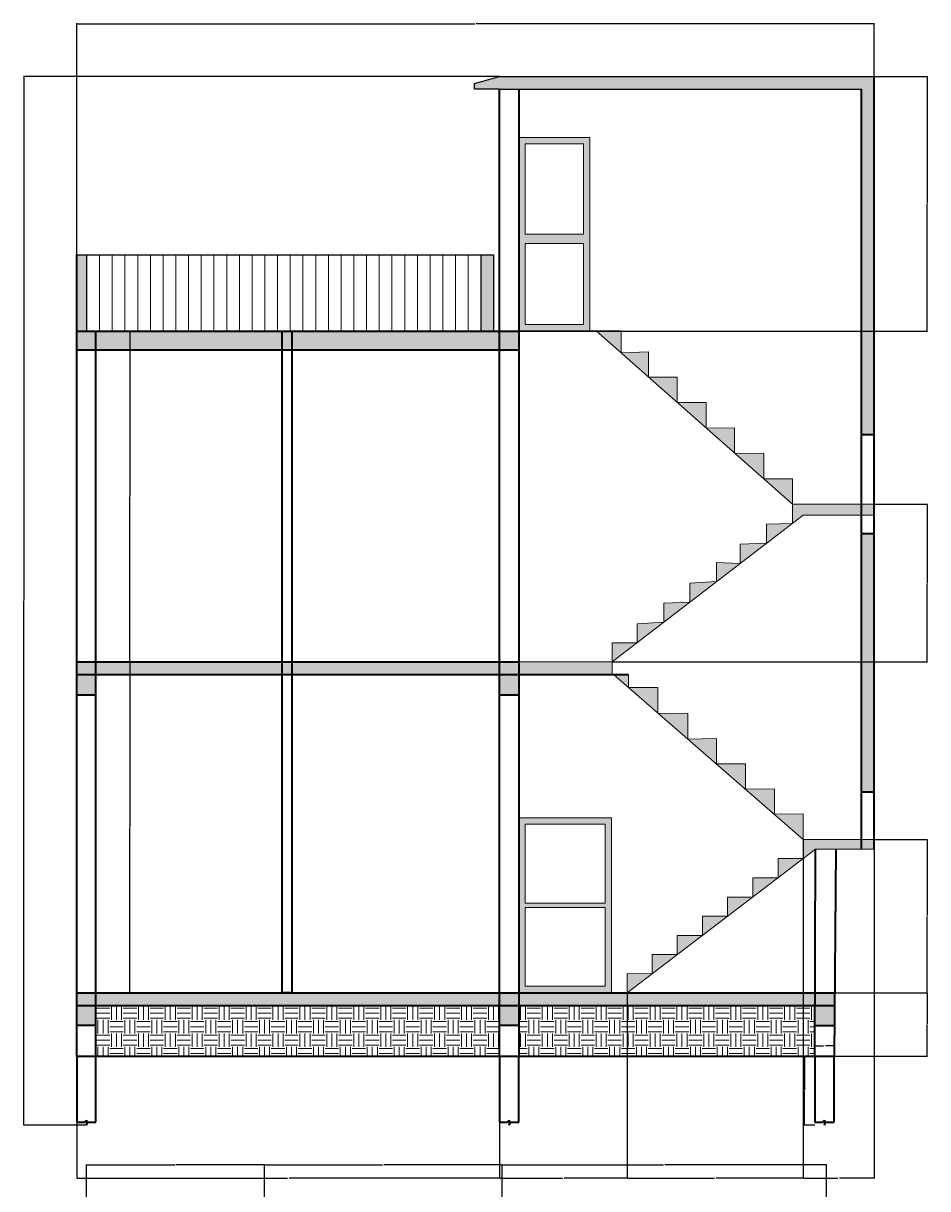
# Model space of a CAD drawing. Units: inches. Extents: x 3504 to 4623, y 2365 to 3357.
# Tile 5 of 5: x 4131 to 4558, y 2803 to 3352. Entities that reach past the tile are written whole.
import ezdxf

# ---------------------------------------------------------------- set-up
doc = ezdxf.new("R2010")
doc.units = ezdxf.units.IN
for name, color, linetype, lineweight in [('A-ANNO-DIMS', 2, 'Continuous', 18), ('A-DOOR', 3, 'Continuous', 18), ('A-FLOR-HRAL', 7, 'Continuous', 25), ('A-FLOR-HRAL-PATT', 252, 'Continuous', 13), ('A-FLOR-STRS', 7, 'Continuous', 18), ('A-ROOF', 7, 'Continuous', 25), ('A-SECT', 7, 'Continuous', 35), ('S-FNDN', 7, 'Continuous', 35)]:
    doc.layers.add(name, color=color, linetype=linetype, lineweight=lineweight)
doc.layers.add('A-SECT-PATT', color=9, linetype='Continuous', lineweight=13, true_color=0xc7c8ca)
doc.layers.add('S-FNDN-PATT', color=9, linetype='Continuous', lineweight=13, true_color=0xc7c8ca)
doc.styles.get("Standard").update_dxf_attribs({"font": 'arial.ttf'})
doc.dimstyles.get("Standard").update_dxf_attribs({"dimtxt": 0.18, "dimasz": 0.18, "dimexe": 0.18, "dimexo": 0.0625, "dimgap": 0.09, "dimtad": 0, "dimtih": 1, "dimtoh": 1, "dimdec": 4, "dimzin": 0, "dimdsep": 46, "dimtxsty": 'Standard', "dimcen": 0.09, "dimadec": 0, "dimazin": 0, "dimtfac": 1, "dimtdec": 4, "dimtofl": 0, "dimtmove": 0, "dimatfit": 3, "dimfxl": 1, "dimtolj": 1, "dimtzin": 0, "dimarcsym": 0})

# ---------------------------------------------------------------- blocks, each defined once
blk = doc.blocks.new('PIER-9-BROKEN-SECTION')
for p, q in [((0, 32.48), (0, 1.39)), ((9, 1.39), (9, 32.48)), ((0, 1.39), (3.55, 1.39)), ((3.55, 1.39), (4.5, 2.34)), ((4.5, 2.34), (4.5, 0)), ((4.5, 0), (5.04, 1.39)), ((5.04, 1.39), (9, 1.39))]:
    blk.add_line(p, q)
blk = doc.blocks.new('*D23')
at = {"layer": 'A-ANNO-DIMS', "color": 0, "lineweight": -2, "transparency": 16777216}
for p, q in [((4504.48, 2864.98), (4499.49, 2864.98)), ((4499.67, 2864.8), (4499.67, 2848.93)), ((4499.67, 2832.69), (4499.67, 2848.56)), ((4504.48, 2832.51), (4499.49, 2832.51))]:
    blk.add_line(p, q, dxfattribs=at)
at = {"layer": 'A-ANNO-DIMS', "color": 0, "transparency": 16777216}
for points in [[(4499.64, 2864.8), (4499.7, 2864.8), (4499.67, 2864.98)], [(4499.64, 2832.69), (4499.7, 2832.69), (4499.67, 2832.51)]]:
    blk.add_solid(points, dxfattribs=at)
at = {"layer": 'Defpoints', "color": 0, "transparency": 16777216}
for p in [(4499.67, 2864.98), (4504.54, 2864.98), (4504.54, 2832.51)]:
    blk.add_point(p, dxfattribs=at)
at = {"layer": 'A-ANNO-DIMS', "color": 0, "transparency": 16777216, "insert": (4499.67, 2848.74), "char_height": 0.18, "attachment_point": 5}
blk.add_mtext('\\A1;PIER 32 TYP.', dxfattribs=at)
blk = doc.blocks.new('*D24')
at = {"layer": 'A-ANNO-DIMS', "color": 0, "lineweight": -2, "transparency": 16777216}
for p, q in [((4504.54, 2865.05), (4504.54, 2870.04)), ((4504.72, 2869.86), (4508.58, 2869.86)), ((4513.36, 2869.86), (4509.5, 2869.86)), ((4513.54, 2865.05), (4513.54, 2870.04))]:
    blk.add_line(p, q, dxfattribs=at)
at = {"layer": 'A-ANNO-DIMS', "color": 0, "transparency": 16777216}
for points in [[(4504.72, 2869.89), (4504.72, 2869.83), (4504.54, 2869.86)], [(4513.36, 2869.89), (4513.36, 2869.83), (4513.54, 2869.86)]]:
    blk.add_solid(points, dxfattribs=at)
at = {"layer": 'Defpoints', "color": 0, "transparency": 16777216}
for p in [(4513.54, 2869.86), (4504.54, 2864.98), (4513.54, 2864.98)]:
    blk.add_point(p, dxfattribs=at)
at = {"layer": 'A-ANNO-DIMS', "color": 0, "transparency": 16777216, "insert": (4509.04, 2869.86), "char_height": 0.18, "attachment_point": 5}
blk.add_mtext('\\A1;9 TYP.', dxfattribs=at)
blk = doc.blocks.new('*D37')
at = {"layer": 'A-ANNO-DIMS', "color": 0, "lineweight": -2, "transparency": 16777216}
for p, q in [((4160.95, 2788.12), (4160.95, 2813.99)), ((4161.13, 2813.81), (4202.73, 2813.81)), ((4244.77, 2813.81), (4203.17, 2813.81)), ((4244.95, 2788.12), (4244.95, 2813.99))]:
    blk.add_line(p, q, dxfattribs=at)
at = {"layer": 'A-ANNO-DIMS', "color": 0, "transparency": 16777216}
for points in [[(4161.13, 2813.84), (4161.13, 2813.78), (4160.95, 2813.81)], [(4244.77, 2813.84), (4244.77, 2813.78), (4244.95, 2813.81)]]:
    blk.add_solid(points, dxfattribs=at)
at = {"layer": 'Defpoints', "color": 0, "transparency": 16777216}
for p in [(4244.95, 2813.81), (4160.95, 2788.06), (4244.95, 2788.06)]:
    blk.add_point(p, dxfattribs=at)
at = {"layer": 'A-ANNO-DIMS', "color": 0, "transparency": 16777216, "insert": (4202.95, 2813.81), "char_height": 0.18, "attachment_point": 5}
blk.add_mtext('\\A1;84', dxfattribs=at)
blk = doc.blocks.new('*D38')
at = {"layer": 'A-ANNO-DIMS', "color": 0, "lineweight": -2, "transparency": 16777216}
for p, q in [((4244.95, 2788.12), (4244.95, 2813.99)), ((4245.13, 2813.81), (4300.67, 2813.81)), ((4356.77, 2813.81), (4301.23, 2813.81)), ((4356.95, 2788.12), (4356.95, 2813.99))]:
    blk.add_line(p, q, dxfattribs=at)
at = {"layer": 'A-ANNO-DIMS', "color": 0, "transparency": 16777216}
for points in [[(4245.13, 2813.84), (4245.13, 2813.78), (4244.95, 2813.81)], [(4356.77, 2813.84), (4356.77, 2813.78), (4356.95, 2813.81)]]:
    blk.add_solid(points, dxfattribs=at)
at = {"layer": 'Defpoints', "color": 0, "transparency": 16777216}
for p in [(4356.95, 2813.81), (4244.95, 2788.06), (4356.95, 2788.06)]:
    blk.add_point(p, dxfattribs=at)
at = {"layer": 'A-ANNO-DIMS', "color": 0, "transparency": 16777216, "insert": (4300.95, 2813.81), "char_height": 0.18, "attachment_point": 5}
blk.add_mtext('\\A1;112', dxfattribs=at)
blk = doc.blocks.new('*D39')
at = {"layer": 'A-ANNO-DIMS', "color": 0, "lineweight": -2, "transparency": 16777216}
for p, q in [((4356.95, 2788.12), (4356.95, 2813.99)), ((4357.13, 2813.81), (4433.17, 2813.81)), ((4509.77, 2813.81), (4433.73, 2813.81)), ((4509.95, 2788.12), (4509.95, 2813.99))]:
    blk.add_line(p, q, dxfattribs=at)
at = {"layer": 'A-ANNO-DIMS', "color": 0, "transparency": 16777216}
for points in [[(4357.13, 2813.84), (4357.13, 2813.78), (4356.95, 2813.81)], [(4509.77, 2813.84), (4509.77, 2813.78), (4509.95, 2813.81)]]:
    blk.add_solid(points, dxfattribs=at)
at = {"layer": 'Defpoints', "color": 0, "transparency": 16777216}
for p in [(4509.95, 2813.81), (4356.95, 2788.06), (4509.95, 2788.06)]:
    blk.add_point(p, dxfattribs=at)
at = {"layer": 'A-ANNO-DIMS', "color": 0, "transparency": 16777216, "insert": (4433.45, 2813.81), "char_height": 0.18, "attachment_point": 5}
blk.add_mtext('\\A1;153', dxfattribs=at)
blk = doc.blocks.new('*D64')
at = {"layer": 'A-ANNO-DIMS', "color": 0, "lineweight": -2, "transparency": 16777216}
for p, q in [((4156.45, 3243.05), (4156.45, 3352.11)), ((4156.63, 3351.93), (4344.16, 3351.93)), ((4532.27, 3351.93), (4344.74, 3351.93)), ((4532.45, 3327.05), (4532.45, 3352.11))]:
    blk.add_line(p, q, dxfattribs=at)
at = {"layer": 'A-ANNO-DIMS', "color": 0, "transparency": 16777216}
for points in [[(4156.63, 3351.96), (4156.63, 3351.9), (4156.45, 3351.93)], [(4532.27, 3351.96), (4532.27, 3351.9), (4532.45, 3351.93)]]:
    blk.add_solid(points, dxfattribs=at)
at = {"layer": 'Defpoints', "color": 0, "transparency": 16777216}
for p in [(4532.45, 3351.93), (4532.45, 3326.98), (4156.45, 3242.98)]:
    blk.add_point(p, dxfattribs=at)
at = {"layer": 'A-ANNO-DIMS', "color": 0, "transparency": 16777216, "insert": (4344.45, 3351.93), "char_height": 0.18, "attachment_point": 5}
blk.add_mtext('\\A1;376', dxfattribs=at)
blk = doc.blocks.new('*D65')
at = {"layer": 'A-ANNO-DIMS', "color": 0, "lineweight": -2, "transparency": 16777216}
for p, q in [((4355.78, 3326.98), (4131.32, 3326.98)), ((4131.5, 3326.8), (4131.5, 3079.93)), ((4131.5, 2832.69), (4131.5, 3079.56)), ((4160.89, 2832.51), (4131.32, 2832.51))]:
    blk.add_line(p, q, dxfattribs=at)
at = {"layer": 'A-ANNO-DIMS', "color": 0, "transparency": 16777216}
for points in [[(4131.47, 3326.8), (4131.53, 3326.8), (4131.5, 3326.98)], [(4131.47, 2832.69), (4131.53, 2832.69), (4131.5, 2832.51)]]:
    blk.add_solid(points, dxfattribs=at)
at = {"layer": 'Defpoints', "color": 0, "transparency": 16777216}
for p in [(4131.5, 3326.98), (4355.84, 3326.98), (4160.95, 2832.51)]:
    blk.add_point(p, dxfattribs=at)
at = {"layer": 'A-ANNO-DIMS', "color": 0, "transparency": 16777216, "insert": (4131.5, 3079.74), "char_height": 0.18, "attachment_point": 5}
blk.add_mtext('\\A1;494.5', dxfattribs=at)
blk = doc.blocks.new('*D66')
at = {"layer": 'A-ANNO-DIMS', "color": 0, "lineweight": -2, "transparency": 16777216}
for p, q in [((4513.88, 2894.98), (4557.58, 2894.98)), ((4557.4, 2894.8), (4557.4, 2880.17)), ((4557.4, 2865.16), (4557.4, 2879.8)), ((4513.6, 2864.98), (4557.58, 2864.98))]:
    blk.add_line(p, q, dxfattribs=at)
at = {"layer": 'A-ANNO-DIMS', "color": 0, "transparency": 16777216}
for points in [[(4557.37, 2894.8), (4557.43, 2894.8), (4557.4, 2894.98)], [(4557.37, 2865.16), (4557.43, 2865.16), (4557.4, 2864.98)]]:
    blk.add_solid(points, dxfattribs=at)
at = {"layer": 'Defpoints', "color": 0, "transparency": 16777216}
for p in [(4513.82, 2894.98), (4557.4, 2894.98), (4513.54, 2864.98)]:
    blk.add_point(p, dxfattribs=at)
at = {"layer": 'A-ANNO-DIMS', "color": 0, "transparency": 16777216, "insert": (4557.4, 2879.98), "char_height": 0.18, "attachment_point": 5}
blk.add_mtext('\\A1;30', dxfattribs=at)
blk = doc.blocks.new('*D67')
at = {"layer": 'A-ANNO-DIMS', "color": 0, "lineweight": -2, "transparency": 16777216}
for p, q in [((4532.51, 2967.25), (4557.58, 2967.25)), ((4557.4, 2967.07), (4557.4, 2931.3)), ((4557.4, 2895.16), (4557.4, 2930.94)), ((4513.88, 2894.98), (4557.58, 2894.98))]:
    blk.add_line(p, q, dxfattribs=at)
at = {"layer": 'A-ANNO-DIMS', "color": 0, "transparency": 16777216}
for points in [[(4557.37, 2967.07), (4557.43, 2967.07), (4557.4, 2967.25)], [(4557.37, 2895.16), (4557.43, 2895.16), (4557.4, 2894.98)]]:
    blk.add_solid(points, dxfattribs=at)
at = {"layer": 'Defpoints', "color": 0, "transparency": 16777216}
for p in [(4532.45, 2967.25), (4557.4, 2967.25), (4513.82, 2894.98)]:
    blk.add_point(p, dxfattribs=at)
at = {"layer": 'A-ANNO-DIMS', "color": 0, "transparency": 16777216, "insert": (4557.4, 2931.12), "char_height": 0.18, "attachment_point": 5}
blk.add_mtext('\\A1;72.27', dxfattribs=at)
blk = doc.blocks.new('*D68')
at = {"layer": 'A-ANNO-DIMS', "color": 0, "lineweight": -2, "transparency": 16777216}
for p, q in [((4156.51, 3050.98), (4181.58, 3050.98)), ((4181.4, 3050.8), (4181.4, 2973.17)), ((4181.4, 2895.16), (4181.4, 2972.8)), ((4156.51, 2894.98), (4181.58, 2894.98))]:
    blk.add_line(p, q, dxfattribs=at)
at = {"layer": 'A-ANNO-DIMS', "color": 0, "transparency": 16777216}
for points in [[(4181.37, 3050.8), (4181.43, 3050.8), (4181.4, 3050.98)], [(4181.37, 2895.16), (4181.43, 2895.16), (4181.4, 2894.98)]]:
    blk.add_solid(points, dxfattribs=at)
at = {"layer": 'Defpoints', "color": 0, "transparency": 16777216}
for p in [(4156.45, 3050.98), (4156.45, 2894.98), (4181.4, 2894.98)]:
    blk.add_point(p, dxfattribs=at)
at = {"layer": 'A-ANNO-DIMS', "color": 0, "transparency": 16777216, "insert": (4181.4, 2972.98), "char_height": 0.18, "attachment_point": 5}
blk.add_mtext('\\A1;156', dxfattribs=at)
blk = doc.blocks.new('*D69')
at = {"layer": 'A-ANNO-DIMS', "color": 0, "lineweight": -2, "transparency": 16777216}
for p, q in [((4156.51, 3206.98), (4181.58, 3206.98)), ((4181.4, 3206.8), (4181.4, 3129.17)), ((4181.4, 3051.16), (4181.4, 3128.8)), ((4156.51, 3050.98), (4181.58, 3050.98))]:
    blk.add_line(p, q, dxfattribs=at)
at = {"layer": 'A-ANNO-DIMS', "color": 0, "transparency": 16777216}
for points in [[(4181.37, 3206.8), (4181.43, 3206.8), (4181.4, 3206.98)], [(4181.37, 3051.16), (4181.43, 3051.16), (4181.4, 3050.98)]]:
    blk.add_solid(points, dxfattribs=at)
at = {"layer": 'Defpoints', "color": 0, "transparency": 16777216}
for p in [(4156.45, 3206.98), (4156.45, 3050.98), (4181.4, 3050.98)]:
    blk.add_point(p, dxfattribs=at)
at = {"layer": 'A-ANNO-DIMS', "color": 0, "transparency": 16777216, "insert": (4181.4, 3128.98), "char_height": 0.18, "attachment_point": 5}
blk.add_mtext('\\A1;156', dxfattribs=at)
blk = doc.blocks.new('*D70')
at = {"layer": 'A-ANNO-DIMS', "color": 0, "lineweight": -2, "transparency": 16777216}
for p, q in [((4532.51, 3125.28), (4557.58, 3125.28)), ((4557.4, 3125.1), (4557.4, 3088.31)), ((4557.4, 3051.16), (4557.4, 3087.95)), ((4408.96, 3050.98), (4557.58, 3050.98))]:
    blk.add_line(p, q, dxfattribs=at)
at = {"layer": 'A-ANNO-DIMS', "color": 0, "transparency": 16777216}
for points in [[(4557.37, 3125.1), (4557.43, 3125.1), (4557.4, 3125.28)], [(4557.37, 3051.16), (4557.43, 3051.16), (4557.4, 3050.98)]]:
    blk.add_solid(points, dxfattribs=at)
at = {"layer": 'Defpoints', "color": 0, "transparency": 16777216}
for p in [(4532.45, 3125.28), (4557.4, 3125.28), (4408.9, 3050.98)]:
    blk.add_point(p, dxfattribs=at)
at = {"layer": 'A-ANNO-DIMS', "color": 0, "transparency": 16777216, "insert": (4557.4, 3088.13), "char_height": 0.18, "attachment_point": 5}
blk.add_mtext('\\A1;74.3', dxfattribs=at)
blk = doc.blocks.new('*D71')
at = {"layer": 'A-ANNO-DIMS', "color": 0, "lineweight": -2, "transparency": 16777216}
for p, q in [((4532.51, 3326.98), (4557.58, 3326.98)), ((4557.4, 3326.8), (4557.4, 3267.17)), ((4557.4, 3207.16), (4557.4, 3266.8)), ((4364.91, 3206.98), (4557.58, 3206.98))]:
    blk.add_line(p, q, dxfattribs=at)
at = {"layer": 'A-ANNO-DIMS', "color": 0, "transparency": 16777216}
for points in [[(4557.37, 3326.8), (4557.43, 3326.8), (4557.4, 3326.98)], [(4557.37, 3207.16), (4557.43, 3207.16), (4557.4, 3206.98)]]:
    blk.add_solid(points, dxfattribs=at)
at = {"layer": 'Defpoints', "color": 0, "transparency": 16777216}
for p in [(4532.45, 3326.98), (4557.4, 3326.98), (4364.84, 3206.98)]:
    blk.add_point(p, dxfattribs=at)
at = {"layer": 'A-ANNO-DIMS', "color": 0, "transparency": 16777216, "insert": (4557.4, 3266.98), "char_height": 0.18, "attachment_point": 5}
blk.add_mtext('\\A1;120', dxfattribs=at)
blk = doc.blocks.new('*D72')
at = {"layer": 'A-ANNO-DIMS', "color": 0, "lineweight": -2, "transparency": 16777216}
for p, q in [((4156.45, 2833.83), (4156.45, 2807.38)), ((4355.84, 2833.83), (4355.84, 2807.38)), ((4156.63, 2807.56), (4255.76, 2807.56)), ((4355.66, 2807.56), (4256.53, 2807.56))]:
    blk.add_line(p, q, dxfattribs=at)
at = {"layer": 'A-ANNO-DIMS', "color": 0, "transparency": 16777216}
for points in [[(4156.63, 2807.59), (4156.63, 2807.53), (4156.45, 2807.56)], [(4355.66, 2807.59), (4355.66, 2807.53), (4355.84, 2807.56)]]:
    blk.add_solid(points, dxfattribs=at)
at = {"layer": 'Defpoints', "color": 0, "transparency": 16777216}
for p in [(4156.45, 2833.9), (4355.84, 2833.9), (4355.84, 2807.56)]:
    blk.add_point(p, dxfattribs=at)
at = {"layer": 'A-ANNO-DIMS', "color": 0, "transparency": 16777216, "insert": (4256.15, 2807.56), "char_height": 0.18, "attachment_point": 5}
blk.add_mtext('\\A1;199.4', dxfattribs=at)
blk = doc.blocks.new('*D73')
at = {"layer": 'A-ANNO-DIMS', "color": 0, "lineweight": -2, "transparency": 16777216}
for p, q in [((4415.96, 2894.92), (4415.96, 2807.38)), ((4355.84, 2833.83), (4355.84, 2807.38)), ((4356.02, 2807.56), (4385.51, 2807.56)), ((4415.78, 2807.56), (4386.3, 2807.56))]:
    blk.add_line(p, q, dxfattribs=at)
at = {"layer": 'A-ANNO-DIMS', "color": 0, "transparency": 16777216}
for points in [[(4356.02, 2807.59), (4356.02, 2807.53), (4355.84, 2807.56)], [(4415.78, 2807.59), (4415.78, 2807.53), (4415.96, 2807.56)]]:
    blk.add_solid(points, dxfattribs=at)
at = {"layer": 'Defpoints', "color": 0, "transparency": 16777216}
for p in [(4415.96, 2894.98), (4355.84, 2833.9), (4415.96, 2807.56)]:
    blk.add_point(p, dxfattribs=at)
at = {"layer": 'A-ANNO-DIMS', "color": 0, "transparency": 16777216, "insert": (4385.9, 2807.56), "char_height": 0.18, "attachment_point": 5}
blk.add_mtext('\\A1;60.12', dxfattribs=at)
blk = doc.blocks.new('*D74')
at = {"layer": 'A-ANNO-DIMS', "color": 0, "lineweight": -2, "transparency": 16777216}
for p, q in [((4499.04, 2967.19), (4499.04, 2807.38)), ((4415.96, 2894.92), (4415.96, 2807.38)), ((4416.14, 2807.56), (4457.11, 2807.56)), ((4498.86, 2807.56), (4457.9, 2807.56))]:
    blk.add_line(p, q, dxfattribs=at)
at = {"layer": 'A-ANNO-DIMS', "color": 0, "transparency": 16777216}
for points in [[(4416.14, 2807.59), (4416.14, 2807.53), (4415.96, 2807.56)], [(4498.86, 2807.59), (4498.86, 2807.53), (4499.04, 2807.56)]]:
    blk.add_solid(points, dxfattribs=at)
at = {"layer": 'Defpoints', "color": 0, "transparency": 16777216}
for p in [(4499.04, 2967.25), (4415.96, 2894.98), (4499.04, 2807.56)]:
    blk.add_point(p, dxfattribs=at)
at = {"layer": 'A-ANNO-DIMS', "color": 0, "transparency": 16777216, "insert": (4457.5, 2807.56), "char_height": 0.18, "attachment_point": 5}
blk.add_mtext('\\A1;83.08', dxfattribs=at)
blk = doc.blocks.new('*D75')
at = {"layer": 'A-ANNO-DIMS', "color": 0, "lineweight": -2, "transparency": 16777216}
for p, q in [((4499.04, 2967.19), (4499.04, 2807.38)), ((4532.45, 2967.19), (4532.45, 2807.38)), ((4499.22, 2807.56), (4515.37, 2807.56)), ((4532.27, 2807.56), (4516.12, 2807.56))]:
    blk.add_line(p, q, dxfattribs=at)
at = {"layer": 'A-ANNO-DIMS', "color": 0, "transparency": 16777216}
for points in [[(4499.22, 2807.59), (4499.22, 2807.53), (4499.04, 2807.56)], [(4532.27, 2807.59), (4532.27, 2807.53), (4532.45, 2807.56)]]:
    blk.add_solid(points, dxfattribs=at)
at = {"layer": 'Defpoints', "color": 0, "transparency": 16777216}
for p in [(4499.04, 2967.25), (4532.45, 2967.25), (4532.45, 2807.56)]:
    blk.add_point(p, dxfattribs=at)
at = {"layer": 'A-ANNO-DIMS', "color": 0, "transparency": 16777216, "insert": (4515.75, 2807.56), "char_height": 0.18, "attachment_point": 5}
blk.add_mtext('\\A1;33.41', dxfattribs=at)

msp = doc.modelspace()

# ---------------------------------------------------------------- hatches: boundary and pattern name
at = {"layer": 'A-FLOR-HRAL-PATT'}
h = msp.add_hatch(dxfattribs=at)
h.set_pattern_fill('ANSI31', color=256, scale=1.888473, angle=45, style=0)
h.paths.add_polyline_path([(4161.3407, 3206.9837), (4346.8407, 3206.9837), (4346.8407, 3242.9837), (4161.3407, 3242.9837)])
at = {"layer": 'A-SECT-PATT'}
h = msp.add_hatch(color=256, dxfattribs=at)
h.dxf.hatch_style = 1
h.paths.add_polyline_path([(4532.4512, 3326.9837), (4355.8429, 3326.9837), (4344.0337, 3323.6736), (4344.0337, 3320.9837), (4355.8429, 3320.9837), (4526.4512, 3320.9837), (4526.4512, 3158.2735), (4532.4512, 3158.2735)])
h.paths.add_polyline_path([(4532.4512, 3111.5685), (4526.4512, 3111.5685), (4526.4512, 2989.6153), (4532.4512, 2989.6153)])
h = msp.add_hatch(color=256, dxfattribs=at)
h.dxf.hatch_style = 1
h.paths.add_polyline_path([(4355.8429, 3050.9837), (4257.7746, 3050.9837), (4257.7746, 3044.9837), (4355.8429, 3044.9837)])
h.paths.add_polyline_path([(4364.8429, 3050.9837), (4355.8429, 3050.9837), (4355.8429, 3044.9837), (4364.8429, 3044.9837)])
h.paths.add_polyline_path([(4408.899, 3050.9837), (4364.8429, 3050.9837), (4364.8429, 3044.9837), (4408.899, 3044.9837)])
h.paths.add_polyline_path([(4257.7746, 3050.9837), (4253.2746, 3050.9837), (4253.2746, 3044.9837), (4257.7746, 3044.9837)])
h.paths.add_polyline_path([(4253.2746, 3050.9837), (4165.4512, 3050.9837), (4165.4512, 3044.9837), (4253.2746, 3044.9837)])
h.paths.add_polyline_path([(4165.4512, 3050.9837), (4156.4512, 3050.9837), (4156.4512, 3044.9837), (4165.4512, 3044.9837)])
h.paths.add_polyline_path([(4165.4512, 2894.9837), (4156.4512, 2894.9837), (4156.4512, 2888.9837), (4165.4512, 2888.9837)])
h.paths.add_polyline_path([(4355.8429, 2894.9837), (4165.4512, 2894.9837), (4165.4512, 2888.9837), (4355.8429, 2888.9837)])
h.paths.add_polyline_path([(4364.8429, 2894.9837), (4355.8429, 2894.9837), (4355.8429, 2888.9837), (4364.8429, 2888.9837)])
h.paths.add_polyline_path([(4504.6335, 2894.9837), (4364.8429, 2894.9837), (4364.8429, 2888.9837), (4504.6144, 2888.9837)])
h.paths.add_polyline_path([(4513.8185, 2894.9837), (4504.6335, 2894.9837), (4504.6144, 2888.9837), (4513.7624, 2888.9837)])
h.paths.add_polyline_path([(4408.6348, 2977.4276), (4364.8429, 2977.4276), (4364.8429, 2894.9837), (4408.6348, 2894.9837)])
h.paths.add_polyline_path([(4367.8429, 2935.2057), (4405.6348, 2935.2057), (4405.6348, 2897.9837), (4367.8429, 2897.9837)], flags=16)
h.paths.add_polyline_path([(4367.8429, 2937.2057), (4367.8429, 2974.4276), (4405.6348, 2974.4276), (4405.6348, 2937.2057)], flags=16)
h.paths.add_polyline_path([(4398.4128, 3298.2205), (4364.8429, 3298.2205), (4364.8429, 3207.1148), (4398.4128, 3207.1148)])
h.paths.add_polyline_path([(4367.8429, 3248.2601), (4395.4128, 3248.2601), (4395.4128, 3210.1148), (4367.8429, 3210.1148)], flags=16)
h.paths.add_polyline_path([(4367.8429, 3252.6677), (4367.8429, 3295.2205), (4395.4128, 3295.2205), (4395.4128, 3252.6677)], flags=16)
h = msp.add_hatch(color=256, dxfattribs=at)
h.dxf.hatch_style = 1
h.paths.add_polyline_path([(4161.0907, 3242.9837), (4156.4512, 3242.9837), (4156.4512, 3206.9837), (4161.0907, 3206.9837)])
h.paths.add_polyline_path([(4353.0907, 3242.9837), (4347.0907, 3242.9837), (4347.0907, 3206.9837), (4353.0907, 3206.9837)])
h = msp.add_hatch(color=256, dxfattribs=at)
h.dxf.hatch_style = 1
h.paths.add_polyline_path([(4165.4512, 3206.9837), (4156.4512, 3206.9837), (4156.4512, 3198.1642), (4165.4512, 3198.1642)])
h.paths.add_polyline_path([(4364.8429, 3206.9837), (4355.8429, 3206.9837), (4355.8429, 3198.1642), (4364.8429, 3198.1642)])
h.paths.add_polyline_path([(4253.2746, 3206.9837), (4165.4512, 3206.9837), (4165.4512, 3198.1642), (4253.2746, 3198.1642)])
h.paths.add_polyline_path([(4355.8429, 3206.9837), (4257.7746, 3206.9837), (4257.7746, 3198.1642), (4355.8429, 3198.1642)])
h.paths.add_polyline_path([(4257.7746, 3206.9837), (4253.2746, 3206.9837), (4253.2746, 3198.1642), (4257.7746, 3198.1642)])
h = msp.add_hatch(color=256, dxfattribs=at)
h.dxf.hatch_style = 1
h.paths.add_polyline_path([(4427.7071, 2903.9276), (4415.962, 2903.9837), (4415.962, 2894.9837)])
h.paths.add_polyline_path([(4439.5365, 2912.9358), (4427.7071, 2912.9276), (4427.7071, 2903.9276)])
h.paths.add_polyline_path([(4451.4327, 2921.9948), (4439.5365, 2921.9358), (4439.5365, 2912.9358)])
h.paths.add_polyline_path([(4463.2767, 2931.014), (4451.4327, 2930.9948), (4451.4327, 2921.9948)])
h.paths.add_polyline_path([(4475.1894, 2940.0856), (4463.2767, 2940.014), (4463.2767, 2931.014)])
h.paths.add_polyline_path([(4487.1592, 2949.2007), (4475.1894, 2949.0856), (4475.1894, 2940.0856)])
h.paths.add_polyline_path([(4499.0443, 2958.2513), (4487.1592, 2958.2007), (4487.1592, 2949.2007)])
h.paths.add_polyline_path([(4504.849, 2962.6715), (4532.4512, 2962.6715), (4532.4512, 2967.2513), (4499.0443, 2967.2513), (4499.0443, 2958.2513)])
h.paths.add_polyline_path([(4499.0443, 2979.2513), (4485.3833, 2979.1242), (4499.0443, 2967.2513)])
h.paths.add_polyline_path([(4485.3833, 2991.1242), (4471.842, 2990.8929), (4485.3833, 2979.1242)])
h.paths.add_polyline_path([(4471.842, 3002.8929), (4458.0908, 3002.8441), (4471.842, 2990.8929)])
h.paths.add_polyline_path([(4458.0908, 3014.8441), (4444.5629, 3014.6012), (4458.0908, 3002.8441)])
h.paths.add_polyline_path([(4444.5629, 3026.6012), (4430.4819, 3026.8391), (4444.5629, 3014.6012)])
h.paths.add_polyline_path([(4430.4819, 3038.8391), (4416.6301, 3038.8777), (4430.4819, 3026.8391)])
h.paths.add_polyline_path([(4416.6301, 3044.9837), (4409.6045, 3044.9837), (4416.6301, 3038.8777)])
h.paths.add_polyline_path([(4420.6327, 3059.9973), (4408.899, 3059.9837), (4408.899, 3050.9837)])
h.paths.add_polyline_path([(4433.2116, 3069.6602), (4420.6327, 3068.9973), (4420.6327, 3059.9973)])
h.paths.add_polyline_path([(4445.5795, 3079.161), (4433.2116, 3078.6602), (4433.2116, 3069.6602)])
h.paths.add_polyline_path([(4458.1322, 3088.8038), (4445.5795, 3088.161), (4445.5795, 3079.161)])
h.paths.add_polyline_path([(4469.3351, 3097.4096), (4458.1322, 3097.8038), (4458.1322, 3088.8038)])
h.paths.add_polyline_path([(4481.7227, 3106.9255), (4469.3351, 3106.4096), (4469.3351, 3097.4096)])
h.paths.add_polyline_path([(4493.8992, 3116.2793), (4481.7227, 3115.9255), (4481.7227, 3106.9255)])
h.paths.add_polyline_path([(4532.4512, 3125.2793), (4493.8992, 3125.2793), (4493.8992, 3116.2793), (4499.0443, 3120.2317), (4532.4512, 3120.2317)])
h.paths.add_polyline_path([(4493.8992, 3137.2793), (4480.3675, 3137.2357), (4493.8992, 3125.2793)])
h.paths.add_polyline_path([(4480.3675, 3149.2357), (4466.6116, 3149.3902), (4480.3675, 3137.2357)])
h.paths.add_polyline_path([(4466.6116, 3161.3902), (4453.1889, 3161.2503), (4466.6116, 3149.3902)])
h.paths.add_polyline_path([(4453.1889, 3173.2503), (4439.5356, 3173.3142), (4453.1889, 3161.2503)])
h.paths.add_polyline_path([(4439.5356, 3185.3142), (4426.0516, 3185.2284), (4439.5356, 3173.3142)])
h.paths.add_polyline_path([(4426.0516, 3197.2284), (4413.1356, 3196.6408), (4426.0516, 3185.2284)])
h.paths.add_polyline_path([(4413.1356, 3207.1148), (4401.2817, 3207.1148), (4413.1356, 3196.6408)])
h = msp.add_hatch(color=256, dxfattribs=at)
h.dxf.hatch_style = 1
h.paths.add_polyline_path([(4165.4512, 3044.9837), (4156.4512, 3044.9837), (4156.4512, 3035.4081), (4165.4512, 3035.4081)])
h.paths.add_polyline_path([(4364.8429, 3044.9837), (4355.8429, 3044.9837), (4355.8429, 3035.4081), (4364.8429, 3035.4081)])
h = msp.add_hatch(color=256, dxfattribs=at)
h.dxf.hatch_style = 1
h.paths.add_polyline_path([(4364.8429, 2888.9837), (4355.8429, 2888.9837), (4355.8429, 2879.518), (4364.8429, 2879.518)])
h.paths.add_polyline_path([(4165.4512, 2888.9837), (4156.4512, 2888.9837), (4156.4512, 2879.518), (4165.4512, 2879.518)])
h.paths.add_polyline_path([(4513.7624, 2888.9837), (4504.6144, 2888.9837), (4504.5843, 2879.518), (4513.6731, 2879.4331)])
at = {"layer": 'S-FNDN-PATT'}
h = msp.add_hatch(dxfattribs=at)
h.set_pattern_fill('EARTH', color=256)
h.paths.add_polyline_path([(4355.8429, 2888.9837), (4165.4512, 2888.9837), (4165.4512, 2864.9837), (4355.8429, 2864.9837)])
h.paths.add_polyline_path([(4504.6144, 2888.9837), (4364.8429, 2888.9837), (4364.8429, 2864.9837), (4504.5381, 2864.9837)])

# ---------------------------------------------------------------- linework, layer by layer
at = {"layer": 'A-DOOR'}
for p, q in [((4364.8429, 3207.1148), (4364.8429, 3298.2205)), ((4364.8429, 3298.2205), (4398.4128, 3298.2205)), ((4398.4128, 3298.2205), (4398.4128, 3207.1148)), ((4367.8429, 3295.2205), (4395.4128, 3295.2205)), ((4367.8429, 3252.6677), (4367.8429, 3295.2205)), ((4395.4128, 3295.2205), (4395.4128, 3252.6677)), ((4367.8429, 3252.6677), (4395.4128, 3252.6677)), ((4367.8429, 3248.2601), (4395.4128, 3248.2601)), ((4367.8429, 3210.1148), (4367.8429, 3248.2601)), ((4395.4128, 3248.2601), (4395.4128, 3210.1148)), ((4395.4128, 3210.1148), (4367.8429, 3210.1148)), ((4398.4128, 3207.1148), (4364.8429, 3207.1148)), ((4398.4128, 3207.1148), (4367.5745, 3207.1148)), ((4367.5745, 3207.1148), (4367.5745, 3207.1148)), ((4367.5745, 3207.1148), (4398.4128, 3207.1148)), ((4398.4128, 3207.1148), (4398.4128, 3207.1148)), ((4367.8429, 2937.2057), (4405.6348, 2937.2057)), ((4367.8429, 2935.2057), (4405.6348, 2935.2057))]:
    msp.add_line(p, q, dxfattribs=at)
msp.add_lwpolyline([(4364.8429, 2894.9837), (4408.6348, 2894.9837), (4408.6348, 2977.4276), (4364.8429, 2977.4276)], close=True, dxfattribs=at)
for points in [[(4405.6348, 2937.2057), (4405.6348, 2974.4276), (4367.8429, 2974.4276), (4367.8429, 2937.2057)], [(4367.8429, 2935.2057), (4367.8429, 2897.9837), (4405.6348, 2897.9837), (4405.6348, 2935.2057)]]:
    msp.add_lwpolyline(points, dxfattribs=at)
at = {"layer": 'A-FLOR-HRAL'}
for p, q in [((4156.4512, 3242.9837), (4353.0907, 3242.9837)), ((4161.0907, 3206.9837), (4161.0907, 3242.9837)), ((4347.0907, 3206.9837), (4347.0907, 3242.9837)), ((4353.0907, 3206.9837), (4353.0907, 3242.9837))]:
    msp.add_line(p, q, dxfattribs=at)
at = {"layer": 'A-FLOR-STRS'}
for p, q in [((4413.1356, 3207.1148), (4364.8429, 3207.1148)), ((4493.8992, 3125.2793), (4401.2817, 3207.1148)), ((4413.1356, 3196.6408), (4413.1356, 3207.1148)), ((4426.0516, 3197.2284), (4413.1356, 3196.6408)), ((4426.0516, 3185.2284), (4426.0516, 3197.2284)), ((4439.5356, 3185.3142), (4426.0516, 3185.2284)), ((4439.5356, 3173.3142), (4439.5356, 3185.3142)), ((4453.1889, 3173.2503), (4439.5356, 3173.3142)), ((4453.1889, 3161.2503), (4453.1889, 3173.2503)), ((4466.6116, 3161.3902), (4453.1889, 3161.2503)), ((4453.1889, 3161.2503), (4453.1889, 3161.2503)), ((4466.6116, 3149.3902), (4466.6116, 3161.3902)), ((4480.3675, 3149.2357), (4466.6116, 3149.3902)), ((4480.3675, 3137.2357), (4480.3675, 3149.2357)), ((4493.8992, 3137.2793), (4480.3675, 3137.2357)), ((4493.8992, 3125.2793), (4493.8992, 3137.2793)), ((4493.8992, 3116.2793), (4493.8992, 3125.2793)), ((4493.8992, 3125.2793), (4532.4512, 3125.2793)), ((4408.899, 3050.9837), (4499.0443, 3120.2317)), ((4481.7227, 3115.9255), (4493.8992, 3116.2793)), ((4499.0443, 3120.2317), (4532.4512, 3120.2317)), ((4481.7227, 3106.9255), (4481.7227, 3115.9255)), ((4469.3351, 3106.4096), (4481.7227, 3106.9255)), ((4469.3351, 3097.4096), (4469.3351, 3106.4096)), ((4458.1322, 3088.8038), (4458.1322, 3097.8038)), ((4458.1322, 3097.8038), (4469.3351, 3097.4096)), ((4445.5795, 3088.161), (4458.1322, 3088.8038)), ((4445.5795, 3079.161), (4445.5795, 3088.161)), ((4433.2116, 3078.6602), (4445.5795, 3079.161)), ((4433.2116, 3069.6602), (4433.2116, 3078.6602)), ((4420.6327, 3068.9973), (4433.2116, 3069.6602)), ((4420.6327, 3059.9973), (4420.6327, 3068.9973)), ((4408.899, 3059.9837), (4420.6327, 3059.9973)), ((4408.899, 3050.9837), (4408.899, 3059.9837)), ((4364.8429, 3050.9837), (4408.899, 3050.9837)), ((4408.899, 3050.9837), (4408.899, 3044.9837)), ((4499.0443, 2967.2513), (4409.6045, 3044.9837)), ((4416.6301, 3044.9837), (4409.6045, 3044.9837)), ((4416.6301, 3038.8777), (4416.6301, 3044.9837)), ((4430.4819, 3038.8391), (4416.6301, 3038.8777)), ((4430.4819, 3026.8391), (4430.4819, 3038.8391)), ((4444.5629, 3026.6012), (4430.4819, 3026.8391)), ((4444.5629, 3014.6012), (4444.5629, 3026.6012)), ((4458.0908, 3014.8441), (4444.5629, 3014.6012)), ((4458.0908, 3002.8441), (4458.0908, 3014.8441)), ((4471.842, 3002.8929), (4458.0908, 3002.8441)), ((4471.842, 2990.8929), (4471.842, 3002.8929)), ((4485.3833, 2991.1242), (4471.842, 2990.8929)), ((4485.3833, 2979.1242), (4485.3833, 2991.1242)), ((4499.0443, 2979.2513), (4485.3833, 2979.1242)), ((4499.0443, 2967.2513), (4499.0443, 2979.2513)), ((4504.849, 2962.6715), (4415.962, 2894.9837)), ((4499.0443, 2958.2513), (4499.0443, 2967.2513)), ((4499.0443, 2967.2513), (4532.4512, 2967.2513)), ((4504.849, 2962.6715), (4532.4512, 2962.6715)), ((4487.1592, 2958.2007), (4499.0443, 2958.2513)), ((4487.1592, 2949.2007), (4487.1592, 2958.2007)), ((4475.1894, 2949.0856), (4487.1592, 2949.2007)), ((4475.1894, 2940.0856), (4475.1894, 2949.0856)), ((4463.2767, 2940.014), (4475.1894, 2940.0856)), ((4463.2767, 2931.014), (4463.2767, 2940.014)), ((4451.4327, 2930.9948), (4463.2767, 2931.014)), ((4451.4327, 2921.9948), (4451.4327, 2930.9948)), ((4439.5365, 2921.9358), (4451.4327, 2921.9948)), ((4439.5365, 2912.9358), (4439.5365, 2921.9358)), ((4427.7071, 2912.9276), (4439.5365, 2912.9358)), ((4427.7071, 2903.9276), (4427.7071, 2912.9276)), ((4415.962, 2894.9837), (4415.962, 2903.9837)), ((4415.962, 2903.9837), (4427.7071, 2903.9276))]:
    msp.add_line(p, q, dxfattribs=at)
at = {"layer": 'A-ROOF'}
for p, q in [((4344.0337, 3323.6736), (4355.8429, 3326.9837)), ((4355.8429, 3326.9837), (4532.4512, 3326.9837)), ((4355.8429, 3326.9837), (4364.8429, 3326.9837)), ((4344.0337, 3320.9837), (4344.0337, 3323.6736)), ((4355.8429, 3320.9837), (4344.0337, 3320.9837)), ((4355.8429, 3320.9837), (4526.4512, 3320.9837))]:
    msp.add_line(p, q, dxfattribs=at)
at = {"layer": 'A-SECT'}
for p, q in [((4532.4512, 2962.6715), (4532.4512, 3326.9837)), ((4355.8429, 2864.9837), (4355.8429, 3320.9837)), ((4364.8429, 3320.9837), (4364.8429, 2864.9837)), ((4526.4512, 2962.6715), (4526.4512, 3320.9837)), ((4156.4512, 2864.9837), (4156.4512, 3242.9837)), ((4156.4512, 3206.9837), (4364.8429, 3206.9837)), ((4165.4512, 2864.9837), (4165.4512, 3206.9837)), ((4253.2746, 2894.9837), (4253.2746, 3206.9837)), ((4253.2746, 3206.9837), (4257.7746, 3206.9837)), ((4257.7746, 3206.9837), (4257.7746, 2894.9837)), ((4156.4512, 3198.1642), (4364.8429, 3198.1642)), ((4526.4512, 3158.2735), (4532.4512, 3158.2735)), ((4526.4512, 3111.5685), (4532.4512, 3111.5685)), ((4156.4512, 3050.9837), (4364.8429, 3050.9837)), ((4156.4512, 3044.9837), (4416.6301, 3044.9837)), ((4156.4512, 3035.4081), (4165.4512, 3035.4081)), ((4355.8429, 3035.4081), (4364.8429, 3035.4081)), ((4526.4512, 2989.6153), (4532.4512, 2989.6153)), ((4504.5381, 2864.9837), (4504.849, 2962.6715)), ((4514.4512, 2962.6715), (4513.5381, 2864.9837)), ((4156.4512, 2894.9837), (4513.8185, 2894.9837)), ((4257.7746, 2894.9837), (4253.2746, 2894.9837)), ((4156.4512, 2888.9837), (4513.7624, 2888.9837)), ((4165.4512, 2879.518), (4156.4512, 2879.518)), ((4364.8429, 2879.518), (4355.8429, 2879.518)), ((4504.5843, 2879.518), (4513.6731, 2879.4331))]:
    msp.add_line(p, q, dxfattribs=at)
at = {"layer": 'S-FNDN'}
msp.add_line((4156.4512, 2864.9837), (4513.5381, 2864.9837), dxfattribs=at)

# ---------------------------------------------------------------- block references
for p in [(4156.4512, 2832.5056), (4355.8429, 2832.5056), (4504.5381, 2832.5056)]:
    msp.add_blockref('PIER-9-BROKEN-SECTION', p, dxfattribs=at)

# ---------------------------------------------------------------- dimensions: what is measured, and where the dimension line sits
at = {"layer": 'A-ANNO-DIMS'}
for base, p1, p2, override, picture, middle in [((4532.4512, 3351.9337), (4156.4512, 3242.9837), (4532.4512, 3326.9837), {"dimdec": 0, "dimlfac": 1, "dimrnd": 0, "dimzin": 0, "dimdsep": 46, "dimlunit": 2}, '*D64', (4344.4512, 3351.9337)), ((4499.0443, 2807.5556), (4415.962, 2894.9837), (4499.0443, 2967.2513), {"dimdec": 2, "dimlfac": 1, "dimrnd": 0, "dimzin": 0, "dimdsep": 46, "dimlunit": 2}, '*D74', (4457.5032, 2807.5556)), ((4532.4512, 2807.5556), (4499.0443, 2967.2513), (4532.4512, 2967.2513), {"dimdec": 2, "dimlfac": 1, "dimrnd": 0, "dimzin": 0, "dimdsep": 46, "dimlunit": 2}, '*D75', (4515.7478, 2807.5556)), ((4415.962, 2807.5556), (4355.8429, 2833.8953), (4415.962, 2894.9837), {"dimdec": 2, "dimlfac": 1, "dimrnd": 0, "dimzin": 0, "dimdsep": 46, "dimlunit": 2}, '*D73', (4385.9025, 2807.5556)), ((4355.8429, 2807.5556), (4156.4512, 2833.8953), (4355.8429, 2833.8953), {"dimdec": 1, "dimlfac": 1, "dimrnd": 0, "dimzin": 0, "dimdsep": 46, "dimlunit": 2}, '*D72', (4256.1471, 2807.5556)), ((4244.9512, 2813.8084), (4160.9512, 2788.0584), (4244.9512, 2788.0584), {"dimdec": 0, "dimlfac": 1, "dimrnd": 0, "dimzin": 0, "dimdsep": 46, "dimlunit": 2}, '*D37', (4202.9512, 2813.8084)), ((4356.9512, 2813.8084), (4244.9512, 2788.0584), (4356.9512, 2788.0584), {"dimdec": 0, "dimlfac": 1, "dimrnd": 0, "dimzin": 0, "dimdsep": 46, "dimlunit": 2}, '*D38', (4300.9512, 2813.8084)), ((4509.9512, 2813.8084), (4356.9512, 2788.0584), (4509.9512, 2788.0584), {"dimdec": 0, "dimlfac": 1, "dimrnd": 0, "dimzin": 0, "dimdsep": 46, "dimlunit": 2}, '*D39', (4433.4512, 2813.8084))]:
    dim = msp.add_linear_dim(base=base, p1=p1, p2=p2, dimstyle='Standard', override=override, dxfattribs=at)
    dim.commit()
    dim.dimension.update_dxf_attribs({"geometry": picture, "text_midpoint": middle})
for base, p1, p2, angle, override, picture, middle in [((4131.5012, 3326.9837), (4160.951, 2832.5056), (4355.8429, 3326.9837), 90, {"dimdec": 1, "dimlfac": 1, "dimrnd": 0, "dimzin": 0, "dimdsep": 46, "dimlunit": 2}, '*D65', (4131.5012, 3079.7447)), ((4557.4012, 3326.9837), (4364.8429, 3206.9837), (4532.4512, 3326.9837), 90, {"dimdec": 0, "dimlfac": 1, "dimrnd": 0, "dimzin": 0, "dimdsep": 46, "dimlunit": 2}, '*D71', (4557.4012, 3266.9837)), ((4181.4012, 3050.9837), (4156.4512, 3206.9837), (4156.4512, 3050.9837), 270, {"dimdec": 0, "dimlfac": 1, "dimrnd": 0, "dimzin": 0, "dimdsep": 46, "dimlunit": 2}, '*D69', (4181.4012, 3128.9837)), ((4557.4012, 3125.2793), (4408.899, 3050.9837), (4532.4512, 3125.2793), 90, {"dimdec": 1, "dimlfac": 1, "dimrnd": 0, "dimzin": 0, "dimdsep": 46, "dimlunit": 2}, '*D70', (4557.4012, 3088.1315)), ((4181.4012, 2894.9837), (4156.4512, 3050.9837), (4156.4512, 2894.9837), 270, {"dimdec": 0, "dimlfac": 1, "dimrnd": 0, "dimzin": 0, "dimdsep": 46, "dimlunit": 2}, '*D68', (4181.4012, 2972.9837)), ((4557.4012, 2967.2513), (4513.8185, 2894.9837), (4532.4512, 2967.2513), 90, {"dimdec": 2, "dimlfac": 1, "dimrnd": 0, "dimzin": 0, "dimdsep": 46, "dimlunit": 2}, '*D67', (4557.4012, 2931.1175)), ((4557.4012, 2894.9837), (4513.5381, 2864.9837), (4513.8185, 2894.9837), 90, {"dimdec": 0, "dimlfac": 1, "dimrnd": 0, "dimzin": 0, "dimdsep": 46, "dimlunit": 2}, '*D66', (4557.4012, 2879.9837))]:
    dim = msp.add_linear_dim(base=base, p1=p1, p2=p2, angle=angle, dimstyle='Standard', override=override, dxfattribs=at)
    dim.commit()
    dim.dimension.update_dxf_attribs({"geometry": picture, "text_midpoint": middle})
dim = msp.add_linear_dim(base=(4513.5381, 2869.8554), p1=(4504.5381, 2864.9837), p2=(4513.5381, 2864.9837), text='<> TYP.', dimstyle='Standard', override={"dimdec": 0, "dimlfac": 1, "dimrnd": 0, "dimzin": 0, "dimdsep": 46, "dimlunit": 2}, dxfattribs=at)
dim.commit()
dim.dimension.update_dxf_attribs({"geometry": '*D24', "text_midpoint": (4509.0381, 2869.8554)})
dim = msp.add_linear_dim(base=(4499.6663, 2864.9837), p1=(4504.5381, 2832.5056), p2=(4504.5381, 2864.9837), angle=90, text='PIER <> TYP.', dimstyle='Standard', override={"dimdec": 0, "dimlfac": 1, "dimrnd": 0, "dimzin": 0, "dimdsep": 46, "dimlunit": 2}, dxfattribs=at)
dim.commit()
dim.dimension.update_dxf_attribs({"geometry": '*D23', "text_midpoint": (4499.6663, 2848.7447)})

doc.saveas('drawing.dxf')
